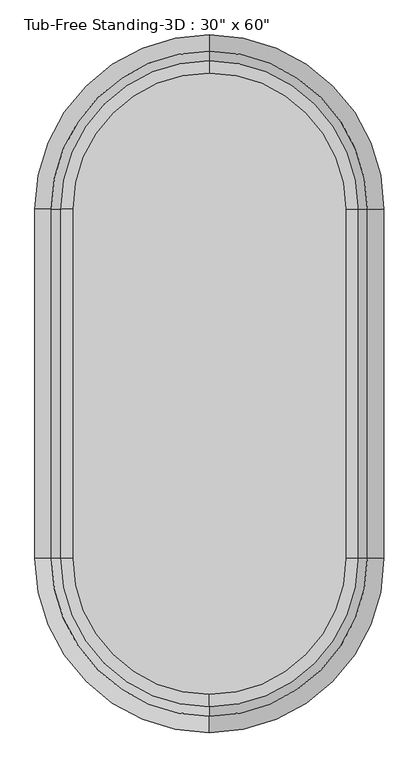
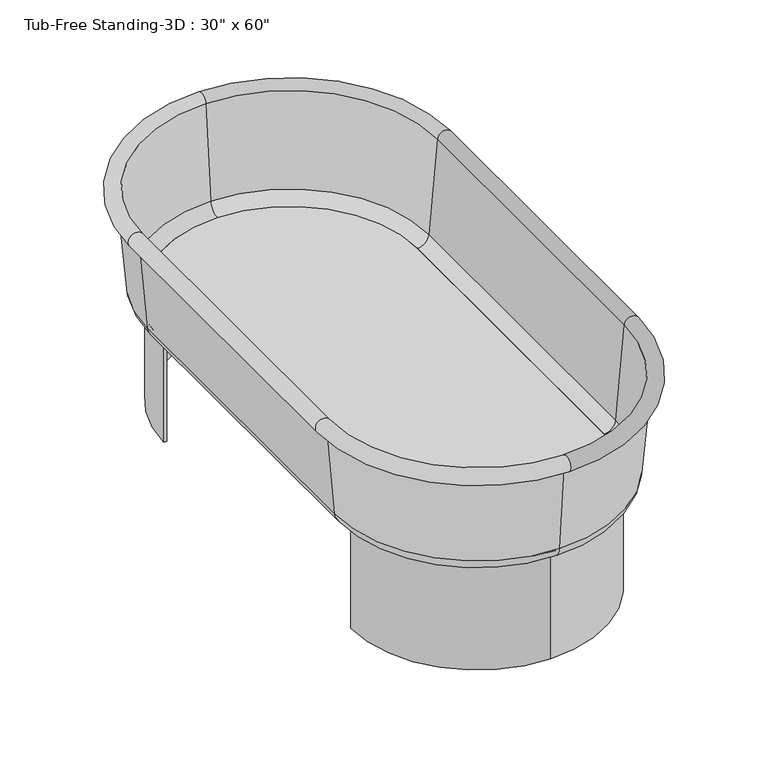
"""IFC4 building model written with IfcOpenShell, lengths in millimetres: flow terminal geometry."""

from ifc_helpers import new_model, si_unit, point, frame, frame_2d, origin, origin_with_axes, place, context, project, spatial, polyline, circle_curve, ellipse_curve, trimmed, segment, composite_curve, outline, extrude, source, transform, mapped, element, save
from ifc_brep_helpers import plane_surface, cylinder_surface, revolved_surface, advanced_brep


def flow_terminal_b46ab875(model_context):
    return source(origin(), model_context, "Body", "SolidModel", [
        extrude(outline(composite_curve([segment(trimmed(circle_curve(frame_2d((0.0, 533.4)), 406.4), [point((0.0, 939.8))], [point((-406.4, 533.4))], True, "CARTESIAN"), True, "CONTINUOUS"), segment(polyline([(-406.4, 533.4), (-416.6824236, 533.4)]), True, "CONTINUOUS"), segment(trimmed(circle_curve(frame_2d((0.0, 533.4)), 416.6824236), [point((-416.6824236, 533.4))], [point((0.0, 950.0824236))], False, "CARTESIAN"), True, "CONTINUOUS"), segment(trimmed(circle_curve(frame_2d((0.0, 533.4)), 416.6824236), [point((0.0, 950.0824236))], [point((416.6824236, 533.4))], False, "CARTESIAN"), True, "CONTINUOUS"), segment(polyline([(416.6824236, 533.4), (406.4, 533.4)]), True, "CONTINUOUS"), segment(trimmed(circle_curve(frame_2d((0.0, 533.4)), 406.4), [point((406.4, 533.4))], [point((0.0, 939.8))], True, "CARTESIAN"), True, "CONTINUOUS")], self_intersect=False)), origin_with_axes(), (0.0, 0.0, 1.0), 368.3),
        extrude(outline(composite_curve([segment(trimmed(circle_curve(frame_2d((0.0, -533.4)), 416.6824236), [point((0.0, -950.0824236))], [point((-416.6824236, -533.4))], False, "CARTESIAN"), True, "CONTINUOUS"), segment(polyline([(-416.6824236, -533.4), (-406.4, -533.4)]), True, "CONTINUOUS"), segment(trimmed(circle_curve(frame_2d((0.0, -533.4)), 406.4), [point((-406.4, -533.4))], [point((0.0, -939.8))], True, "CARTESIAN"), True, "CONTINUOUS"), segment(trimmed(circle_curve(frame_2d((0.0, -533.4)), 406.4), [point((0.0, -939.8))], [point((406.4, -533.4))], True, "CARTESIAN"), True, "CONTINUOUS"), segment(polyline([(406.4, -533.4), (416.6824236, -533.4)]), True, "CONTINUOUS"), segment(trimmed(circle_curve(frame_2d((0.0, -533.4)), 416.6824236), [point((416.6824236, -533.4))], [point((0.0, -950.0824236))], False, "CARTESIAN"), True, "CONTINUOUS")], self_intersect=False)), origin_with_axes(), (0.0, 0.0, 1.0), 368.3),
        extrude(outline(composite_curve([segment(polyline([(-416.6824236, -533.4), (-416.6824236, 533.4)]), True, "CONTINUOUS"), segment(trimmed(circle_curve(frame_2d((0.0, 533.4)), 416.6824236), [point((-416.6824236, 533.4))], [point((0.0, 950.0824236))], False, "CARTESIAN"), True, "CONTINUOUS"), segment(trimmed(circle_curve(frame_2d((0.0, 533.4)), 416.6824236), [point((0.0, 950.0824236))], [point((416.6824236, 533.4))], False, "CARTESIAN"), True, "CONTINUOUS"), segment(polyline([(416.6824236, 533.4), (416.6824236, -533.4)]), True, "CONTINUOUS"), segment(trimmed(circle_curve(frame_2d((0.0, -533.4)), 416.6824236), [point((416.6824236, -533.4))], [point((0.0, -950.0824236))], False, "CARTESIAN"), True, "CONTINUOUS"), segment(trimmed(circle_curve(frame_2d((0.0, -533.4)), 416.6824236), [point((0.0, -950.0824236))], [point((-416.6824236, -533.4))], False, "CARTESIAN"), True, "CONTINUOUS")], self_intersect=False)), frame((0.0, 0.0, 368.3), z_axis=(0.0, 0.0, 1.0), x_axis=(1.0, 0.0, 0.0)), (0.0, 0.0, 1.0), 15.08125),
        advanced_brep(
        [(0.0, -1028.7, 711.2), (495.3, -533.4, 711.2), (508.0, -533.4, 711.2), (0.0, -1041.4, 711.2), (0.0, -1002.9045038, 416.3561295), (469.5045038, -533.4, 416.3561295), (0.0, -950.0824236, 367.9536107), (416.6824236, -533.4, 367.9536107), (0.0, -950.0824236, 382.8774627), (416.6824236, -533.4, 382.8774627), (0.0, -988.0374416, 417.6568289), (454.6374416, -533.4, 417.6568289), (0.0, -1016.2561556, 740.1982063), (482.8561556, -533.4, 740.1982063), (-495.3, -533.4, 711.2), (-508.0, -533.4, 711.2), (-469.5045038, -533.4, 416.3561295), (-416.6824236, -533.4, 367.9536107), (-416.6824236, -533.4, 382.8774627), (-454.6374416, -533.4, 417.6568289), (-482.8561556, -533.4, 740.1982063), (-508.0, 533.4, 711.2), (-495.3, 533.4, 711.2), (-469.5045038, 533.4, 416.3561295), (-416.6824236, 533.4, 367.9536107), (-416.6824236, 533.4, 382.8774627), (-454.6374416, 533.4, 417.6568289), (-482.8561556, 533.4, 740.1982063), (0.0, 1028.7, 711.2), (0.0, 1041.4, 711.2), (0.0, 1002.9045038, 416.3561295), (0.0, 950.0824236, 367.9536107), (0.0, 950.0824236, 382.8774627), (0.0, 988.0374416, 417.6568289), (0.0, 1016.2561556, 740.1982063), (495.3, 533.4, 711.2), (508.0, 533.4, 711.2), (469.5045038, 533.4, 416.3561295), (416.6824236, 533.4, 367.9536107), (416.6824236, 533.4, 382.8774627), (454.6374416, 533.4, 417.6568289), (482.8561556, 533.4, 740.1982063)],
        [
            (0, 1, circle_curve(frame((0.0, -533.4, 711.2), z_axis=(0.0, 0.0, 1.0), x_axis=(1.0, 0.0, 0.0)), 495.3)),
            (1, 2),
            (2, 3, circle_curve(frame((0.0, -533.4, 711.2), z_axis=(0.0, 0.0, -1.0), x_axis=(1.0, 0.0, 0.0)), 508.0)),
            (3, 0),
            (4, 5, circle_curve(frame((0.0, -533.4, 416.3561295), z_axis=(0.0, 0.0, 1.0), x_axis=(1.0, 0.0, 0.0)), 469.5045038)),
            (5, 1),
            (0, 4),
            (6, 7, circle_curve(frame((0.0, -533.4, 367.9536107), z_axis=(0.0, 0.0, 1.0), x_axis=(1.0, 0.0, 0.0)), 416.6824236)),
            (7, 5, circle_curve(frame((416.6824236, -533.4, 420.9774627), z_axis=(0.0, -1.0, 0.0), x_axis=(1.0, 0.0, 0.0)), 53.023852)),
            (4, 6, circle_curve(frame((0.0, -950.0824236, 420.9774627), z_axis=(1.0, 0.0, 0.0), x_axis=(0.0, -1.0, 0.0)), 53.023852)),
            (8, 9, circle_curve(frame((0.0, -533.4, 382.8774627), z_axis=(0.0, 0.0, 1.0), x_axis=(1.0, 0.0, 0.0)), 416.6824236)),
            (9, 7),
            (6, 8),
            (10, 11, circle_curve(frame((0.0, -533.4, 417.6568289), z_axis=(0.0, 0.0, 1.0), x_axis=(1.0, 0.0, 0.0)), 454.6374416)),
            (11, 9, circle_curve(frame((416.6824236, -533.4, 420.9774627), z_axis=(0.0, 1.0, 0.0), x_axis=(1.0, 0.0, 0.0)), 38.1)),
            (8, 10, circle_curve(frame((0.0, -950.0824236, 420.9774627), z_axis=(-1.0, 0.0, 0.0), x_axis=(0.0, -1.0, 0.0)), 38.1)),
            (12, 13, circle_curve(frame((0.0, -533.4, 740.1982063), z_axis=(0.0, 0.0, 1.0), x_axis=(1.0, 0.0, 0.0)), 482.8561556)),
            (13, 11),
            (10, 12),
            (2, 13, circle_curve(frame((508.0, -533.4, 736.6), z_axis=(0.0, -1.0, 0.0), x_axis=(1.0, 0.0, 0.0)), 25.4)),
            (12, 3, circle_curve(frame((0.0, -1041.4, 736.6), z_axis=(1.0, 0.0, 0.0), x_axis=(0.0, -1.0, 0.0)), 25.4)),
            (14, 0, circle_curve(frame((0.0, -533.4, 711.2), z_axis=(0.0, 0.0, 1.0), x_axis=(0.0, -1.0, 0.0)), 495.3)),
            (3, 15, circle_curve(frame((0.0, -533.4, 711.2), z_axis=(0.0, 0.0, -1.0), x_axis=(0.0, -1.0, 0.0)), 508.0)),
            (15, 14),
            (16, 4, circle_curve(frame((0.0, -533.4, 416.3561295), z_axis=(0.0, 0.0, 1.0), x_axis=(0.0, -1.0, 0.0)), 469.5045038)),
            (14, 16),
            (17, 6, circle_curve(frame((0.0, -533.4, 367.9536107), z_axis=(0.0, 0.0, 1.0), x_axis=(0.0, -1.0, 0.0)), 416.6824236)),
            (16, 17, circle_curve(frame((-416.6824236, -533.4, 420.9774627), z_axis=(0.0, -1.0, 0.0), x_axis=(-1.0, 0.0, 0.0)), 53.023852)),
            (18, 8, circle_curve(frame((0.0, -533.4, 382.8774627), z_axis=(0.0, 0.0, 1.0), x_axis=(0.0, -1.0, 0.0)), 416.6824236)),
            (17, 18),
            (19, 10, circle_curve(frame((0.0, -533.4, 417.6568289), z_axis=(0.0, 0.0, 1.0), x_axis=(0.0, -1.0, 0.0)), 454.6374416)),
            (18, 19, circle_curve(frame((-416.6824236, -533.4, 420.9774627), z_axis=(0.0, 1.0, 0.0), x_axis=(-1.0, 0.0, 0.0)), 38.1)),
            (20, 12, circle_curve(frame((0.0, -533.4, 740.1982063), z_axis=(0.0, 0.0, 1.0), x_axis=(0.0, -1.0, 0.0)), 482.8561556)),
            (19, 20),
            (20, 15, circle_curve(frame((-508.0, -533.4, 736.6), z_axis=(0.0, -1.0, 0.0), x_axis=(-1.0, 0.0, 0.0)), 25.4)),
            (15, 21),
            (21, 22),
            (22, 14),
            (22, 23),
            (23, 16),
            (23, 24, circle_curve(frame((-416.6824236, 533.4, 420.9774627), z_axis=(0.0, -1.0, 0.0), x_axis=(-1.0, 0.0, 0.0)), 53.023852)),
            (24, 17),
            (24, 25),
            (25, 18),
            (25, 26, circle_curve(frame((-416.6824236, 533.4, 420.9774627), z_axis=(0.0, 1.0, 0.0), x_axis=(-1.0, 0.0, 0.0)), 38.1)),
            (26, 19),
            (26, 27),
            (27, 20),
            (27, 21, circle_curve(frame((-508.0, 533.4, 736.6), z_axis=(0.0, -1.0, 0.0), x_axis=(-1.0, 0.0, 0.0)), 25.4)),
            (28, 22, circle_curve(frame((0.0, 533.4, 711.2), z_axis=(0.0, 0.0, 1.0), x_axis=(-1.0, 0.0, 0.0)), 495.3)),
            (21, 29, circle_curve(frame((0.0, 533.4, 711.2), z_axis=(0.0, 0.0, -1.0), x_axis=(-1.0, 0.0, 0.0)), 508.0)),
            (29, 28),
            (30, 23, circle_curve(frame((0.0, 533.4, 416.3561295), z_axis=(0.0, 0.0, 1.0), x_axis=(-1.0, 0.0, 0.0)), 469.5045038)),
            (28, 30),
            (31, 24, circle_curve(frame((0.0, 533.4, 367.9536107), z_axis=(0.0, 0.0, 1.0), x_axis=(-1.0, 0.0, 0.0)), 416.6824236)),
            (30, 31, circle_curve(frame((0.0, 950.0824236, 420.9774627), z_axis=(-1.0, 0.0, 0.0), x_axis=(0.0, 1.0, 0.0)), 53.023852)),
            (32, 25, circle_curve(frame((0.0, 533.4, 382.8774627), z_axis=(0.0, 0.0, 1.0), x_axis=(-1.0, 0.0, 0.0)), 416.6824236)),
            (31, 32),
            (33, 26, circle_curve(frame((0.0, 533.4, 417.6568289), z_axis=(0.0, 0.0, 1.0), x_axis=(-1.0, 0.0, 0.0)), 454.6374416)),
            (32, 33, circle_curve(frame((0.0, 950.0824236, 420.9774627), z_axis=(1.0, 0.0, 0.0), x_axis=(0.0, 1.0, 0.0)), 38.1)),
            (34, 27, circle_curve(frame((0.0, 533.4, 740.1982063), z_axis=(0.0, 0.0, 1.0), x_axis=(-1.0, 0.0, 0.0)), 482.8561556)),
            (33, 34),
            (34, 29, circle_curve(frame((0.0, 1041.4, 736.6), z_axis=(-1.0, 0.0, 0.0), x_axis=(0.0, 1.0, 0.0)), 25.4)),
            (35, 28, circle_curve(frame((0.0, 533.4, 711.2), z_axis=(0.0, 0.0, 1.0), x_axis=(0.0, 1.0, 0.0)), 495.3)),
            (29, 36, circle_curve(frame((0.0, 533.4, 711.2), z_axis=(0.0, 0.0, -1.0), x_axis=(0.0, 1.0, 0.0)), 508.0)),
            (36, 35),
            (37, 30, circle_curve(frame((0.0, 533.4, 416.3561295), z_axis=(0.0, 0.0, 1.0), x_axis=(0.0, 1.0, 0.0)), 469.5045038)),
            (35, 37),
            (38, 31, circle_curve(frame((0.0, 533.4, 367.9536107), z_axis=(0.0, 0.0, 1.0), x_axis=(0.0, 1.0, 0.0)), 416.6824236)),
            (37, 38, circle_curve(frame((416.6824236, 533.4, 420.9774627), z_axis=(0.0, 1.0, 0.0), x_axis=(1.0, 0.0, 0.0)), 53.023852)),
            (39, 32, circle_curve(frame((0.0, 533.4, 382.8774627), z_axis=(0.0, 0.0, 1.0), x_axis=(0.0, 1.0, 0.0)), 416.6824236)),
            (38, 39),
            (40, 33, circle_curve(frame((0.0, 533.4, 417.6568289), z_axis=(0.0, 0.0, 1.0), x_axis=(0.0, 1.0, 0.0)), 454.6374416)),
            (39, 40, circle_curve(frame((416.6824236, 533.4, 420.9774627), z_axis=(0.0, -1.0, 0.0), x_axis=(1.0, 0.0, 0.0)), 38.1)),
            (41, 34, circle_curve(frame((0.0, 533.4, 740.1982063), z_axis=(0.0, 0.0, 1.0), x_axis=(0.0, 1.0, 0.0)), 482.8561556)),
            (40, 41),
            (41, 36, circle_curve(frame((508.0, 533.4, 736.6), z_axis=(0.0, 1.0, 0.0), x_axis=(1.0, 0.0, 0.0)), 25.4)),
            (36, 2),
            (1, 35),
            (5, 37),
            (7, 38),
            (9, 39),
            (11, 40),
            (13, 41),
        ],
        [
            plane_surface(frame((0.0, -533.4, 711.2), z_axis=(0.0, 0.0, -1.0), x_axis=(1.0, 0.0, 0.0))),
            revolved_surface(polyline([(495.3, -533.4, 711.2), (469.5045038, -533.4, 416.3561295)]), (0.0, -533.4, 736.6), (0.0, 0.0, -1.0)),
            revolved_surface(trimmed(ellipse_curve(frame((416.6824236, -533.4, 420.9774627), z_axis=(0.0, 1.0, 0.0), x_axis=(1.0, 0.0, 0.0)), 53.023852, 53.023852), [point((469.5045038, -533.4, 416.3561295))], [point((416.6824236, -533.4, 367.9536107))], True, "CARTESIAN"), (0.0, -533.4, 736.6), (0.0, 0.0, -1.0)),
            revolved_surface(polyline([(416.6824236, -533.4, 367.9536107), (416.6824236, -533.4, 382.8774627)]), (0.0, -533.4, 736.6), (0.0, 0.0, -1.0)),
            revolved_surface(trimmed(ellipse_curve(frame((416.6824236, -533.4, 420.9774627), z_axis=(0.0, -1.0, 0.0), x_axis=(1.0, 0.0, 0.0)), 38.1, 38.1), [point((416.6824236, -533.4, 382.8774627))], [point((454.6374416, -533.4, 417.6568289))], True, "CARTESIAN"), (0.0, -533.4, 736.6), (0.0, 0.0, -1.0)),
            revolved_surface(polyline([(454.6374416, -533.4, 417.6568289), (482.8561556, -533.4, 740.1982063)]), (0.0, -533.4, 736.6), (0.0, 0.0, -1.0)),
            revolved_surface(trimmed(ellipse_curve(frame((508.0, -533.4, 736.6), z_axis=(0.0, 1.0, 0.0), x_axis=(1.0, 0.0, 0.0)), 25.4, 25.4), [point((482.8561556, -533.4, 740.1982063))], [point((508.0, -533.4, 711.2))], True, "CARTESIAN"), (0.0, -533.4, 736.6), (0.0, 0.0, -1.0)),
            plane_surface(frame((0.0, -533.4, 711.2), z_axis=(0.0, 0.0, -1.0), x_axis=(0.0, -1.0, 0.0))),
            revolved_surface(polyline([(0.0, -1028.7, 711.2), (0.0, -1002.9045038, 416.3561295)]), (0.0, -533.4, 736.6), (0.0, 0.0, -1.0)),
            revolved_surface(trimmed(ellipse_curve(frame((0.0, -950.0824236, 420.9774627), z_axis=(1.0, 0.0, 0.0), x_axis=(0.0, -1.0, 0.0)), 53.023852, 53.023852), [point((0.0, -1002.9045038, 416.3561295))], [point((0.0, -950.0824236, 367.9536107))], True, "CARTESIAN"), (0.0, -533.4, 736.6), (0.0, 0.0, -1.0)),
            revolved_surface(polyline([(0.0, -950.0824236, 367.9536107), (0.0, -950.0824236, 382.8774627)]), (0.0, -533.4, 736.6), (0.0, 0.0, -1.0)),
            revolved_surface(trimmed(ellipse_curve(frame((0.0, -950.0824236, 420.9774627), z_axis=(-1.0, 0.0, 0.0), x_axis=(0.0, -1.0, 0.0)), 38.1, 38.1), [point((0.0, -950.0824236, 382.8774627))], [point((0.0, -988.0374416, 417.6568289))], True, "CARTESIAN"), (0.0, -533.4, 736.6), (0.0, 0.0, -1.0)),
            revolved_surface(polyline([(0.0, -988.0374416, 417.6568289), (0.0, -1016.2561556, 740.1982063)]), (0.0, -533.4, 736.6), (0.0, 0.0, -1.0)),
            revolved_surface(trimmed(ellipse_curve(frame((0.0, -1041.4, 736.6), z_axis=(1.0, 0.0, 0.0), x_axis=(0.0, -1.0, 0.0)), 25.4, 25.4), [point((0.0, -1016.2561556, 740.1982063))], [point((0.0, -1041.4, 711.2))], True, "CARTESIAN"), (0.0, -533.4, 736.6), (0.0, 0.0, -1.0)),
            plane_surface(frame((-508.0, -533.4, 711.2), z_axis=(0.0, 0.0, -1.0), x_axis=(0.0, 1.0, 0.0))),
            plane_surface(frame((-495.3, -533.4, 711.2), z_axis=(-0.9961946980917455, 0.0, -0.0871557427476588), x_axis=(0.0, 1.0, 0.0))),
            cylinder_surface(frame((-416.6824236, -533.4, 420.9774627), z_axis=(0.0, -1.0, 0.0), x_axis=(-1.0, 0.0, 0.0)), 53.023852),
            plane_surface(frame((-416.6824236, -533.4, 367.9536107), z_axis=(1.0, 0.0, 0.0), x_axis=(0.0, 1.0, 0.0))),
            revolved_surface(polyline([(-454.7824236, 533.4, 420.9774627), (-454.7824236, -533.4, 420.9774627)]), (-416.6824236, -533.4, 420.9774627), (0.0, 1.0, 0.0)),
            plane_surface(frame((-454.6374416, -533.4, 417.6568289), z_axis=(0.9961946980917457, 0.0, 0.08715574274765674), x_axis=(0.0, 1.0, 0.0))),
            cylinder_surface(frame((-508.0, -533.4, 736.6), z_axis=(0.0, -1.0, 0.0), x_axis=(-1.0, 0.0, 0.0)), 25.4),
            plane_surface(frame((0.0, 533.4, 711.2), z_axis=(0.0, 0.0, -1.0), x_axis=(-1.0, 0.0, 0.0))),
            revolved_surface(polyline([(-495.3, 533.4, 711.2), (-469.5045038, 533.4, 416.3561295)]), (0.0, 533.4, 736.6), (0.0, 0.0, -1.0)),
            revolved_surface(trimmed(ellipse_curve(frame((-416.6824236, 533.4, 420.9774627), z_axis=(0.0, -1.0, 0.0), x_axis=(-1.0, 0.0, 0.0)), 53.023852, 53.023852), [point((-469.5045038, 533.4, 416.3561295))], [point((-416.6824236, 533.4, 367.9536107))], True, "CARTESIAN"), (0.0, 533.4, 736.6), (0.0, 0.0, -1.0)),
            revolved_surface(polyline([(-416.6824236, 533.4, 367.9536107), (-416.6824236, 533.4, 382.8774627)]), (0.0, 533.4, 736.6), (0.0, 0.0, -1.0)),
            revolved_surface(trimmed(ellipse_curve(frame((-416.6824236, 533.4, 420.9774627), z_axis=(0.0, 1.0, 0.0), x_axis=(-1.0, 0.0, 0.0)), 38.1, 38.1), [point((-416.6824236, 533.4, 382.8774627))], [point((-454.6374416, 533.4, 417.6568289))], True, "CARTESIAN"), (0.0, 533.4, 736.6), (0.0, 0.0, -1.0)),
            revolved_surface(polyline([(-454.6374416, 533.4, 417.6568289), (-482.8561556, 533.4, 740.1982063)]), (0.0, 533.4, 736.6), (0.0, 0.0, -1.0)),
            revolved_surface(trimmed(ellipse_curve(frame((-508.0, 533.4, 736.6), z_axis=(0.0, -1.0, 0.0), x_axis=(-1.0, 0.0, 0.0)), 25.4, 25.4), [point((-482.8561556, 533.4, 740.1982063))], [point((-508.0, 533.4, 711.2))], True, "CARTESIAN"), (0.0, 533.4, 736.6), (0.0, 0.0, -1.0)),
            plane_surface(frame((0.0, 533.4, 711.2), z_axis=(0.0, 0.0, -1.0), x_axis=(0.0, 1.0, 0.0))),
            revolved_surface(polyline([(0.0, 1028.7, 711.2), (0.0, 1002.9045038, 416.3561295)]), (0.0, 533.4, 736.6), (0.0, 0.0, -1.0)),
            revolved_surface(trimmed(ellipse_curve(frame((0.0, 950.0824236, 420.9774627), z_axis=(-1.0, 0.0, 0.0), x_axis=(0.0, 1.0, 0.0)), 53.023852, 53.023852), [point((0.0, 1002.9045038, 416.3561295))], [point((0.0, 950.0824236, 367.9536107))], True, "CARTESIAN"), (0.0, 533.4, 736.6), (0.0, 0.0, -1.0)),
            revolved_surface(polyline([(0.0, 950.0824236, 367.9536107), (0.0, 950.0824236, 382.8774627)]), (0.0, 533.4, 736.6), (0.0, 0.0, -1.0)),
            revolved_surface(trimmed(ellipse_curve(frame((0.0, 950.0824236, 420.9774627), z_axis=(1.0, 0.0, 0.0), x_axis=(0.0, 1.0, 0.0)), 38.1, 38.1), [point((0.0, 950.0824236, 382.8774627))], [point((0.0, 988.0374416, 417.6568289))], True, "CARTESIAN"), (0.0, 533.4, 736.6), (0.0, 0.0, -1.0)),
            revolved_surface(polyline([(0.0, 988.0374416, 417.6568289), (0.0, 1016.2561556, 740.1982063)]), (0.0, 533.4, 736.6), (0.0, 0.0, -1.0)),
            revolved_surface(trimmed(ellipse_curve(frame((0.0, 1041.4, 736.6), z_axis=(-1.0, 0.0, 0.0), x_axis=(0.0, 1.0, 0.0)), 25.4, 25.4), [point((0.0, 1016.2561556, 740.1982063))], [point((0.0, 1041.4, 711.2))], True, "CARTESIAN"), (0.0, 533.4, 736.6), (0.0, 0.0, -1.0)),
            plane_surface(frame((508.0, 533.4, 711.2), z_axis=(0.0, 0.0, -1.0), x_axis=(0.0, -1.0, 0.0))),
            plane_surface(frame((495.3, 533.4, 711.2), z_axis=(0.9961946980917455, 0.0, -0.0871557427476588), x_axis=(0.0, -1.0, 0.0))),
            cylinder_surface(frame((416.6824236, 533.4, 420.9774627), z_axis=(0.0, 1.0, 0.0), x_axis=(1.0, 0.0, 0.0)), 53.023852),
            plane_surface(frame((416.6824236, 533.4, 367.9536107), z_axis=(-1.0, 0.0, 0.0), x_axis=(0.0, -1.0, 0.0))),
            revolved_surface(polyline([(454.7824236, -533.4, 420.9774627), (454.7824236, 533.4, 420.9774627)]), (416.6824236, 533.4, 420.9774627), (0.0, -1.0, 0.0)),
            plane_surface(frame((454.6374416, 533.4, 417.6568289), z_axis=(-0.9961946980917458, 0.0, 0.08715574274765675), x_axis=(0.0, -1.0, 0.0))),
            cylinder_surface(frame((508.0, 533.4, 736.6), z_axis=(0.0, 1.0, 0.0), x_axis=(1.0, 0.0, 0.0)), 25.4),
        ],
        [
            (0, [[1, 2, 3, 4]]),
            (1, [[5, 6, -1, 7]]),
            (2, [[8, 9, -5, 10]]),
            (3, [[11, 12, -8, 13]]),
            (4, [[14, 15, -11, 16]]),
            (5, [[17, 18, -14, 19]]),
            (6, [[-3, 20, -17, 21]]),
            (7, [[22, -4, 23, 24]]),
            (8, [[25, -7, -22, 26]]),
            (9, [[27, -10, -25, 28]]),
            (10, [[29, -13, -27, 30]]),
            (11, [[31, -16, -29, 32]]),
            (12, [[33, -19, -31, 34]]),
            (13, [[-23, -21, -33, 35]]),
            (14, [[-24, 36, 37, 38]]),
            (15, [[-26, -38, 39, 40]]),
            (16, [[-28, -40, 41, 42]]),
            (17, [[-30, -42, 43, 44]]),
            (18, [[-32, -44, 45, 46]]),
            (19, [[-34, -46, 47, 48]]),
            (20, [[-35, -48, 49, -36]]),
            (21, [[50, -37, 51, 52]]),
            (22, [[53, -39, -50, 54]]),
            (23, [[55, -41, -53, 56]]),
            (24, [[57, -43, -55, 58]]),
            (25, [[59, -45, -57, 60]]),
            (26, [[61, -47, -59, 62]]),
            (27, [[-51, -49, -61, 63]]),
            (28, [[64, -52, 65, 66]]),
            (29, [[67, -54, -64, 68]]),
            (30, [[69, -56, -67, 70]]),
            (31, [[71, -58, -69, 72]]),
            (32, [[73, -60, -71, 74]]),
            (33, [[75, -62, -73, 76]]),
            (34, [[-65, -63, -75, 77]]),
            (35, [[-66, 78, -2, 79]]),
            (36, [[-68, -79, -6, 80]]),
            (37, [[-70, -80, -9, 81]]),
            (38, [[-72, -81, -12, 82]]),
            (39, [[-74, -82, -15, 83]]),
            (40, [[-76, -83, -18, 84]]),
            (41, [[-77, -84, -20, -78]]),
        ],
    ),
    ])


if __name__ == "__main__":
    model = new_model("IFC4")
    model_context = context("Model", 3, world=origin())
    ifc_project = project(units=[si_unit("LENGTHUNIT", "METRE", prefix="MILLI")], contexts=[model_context])
    site = spatial("IfcSite", under=ifc_project)
    building = spatial("IfcBuilding", under=site)
    placement = place(None, origin())
    flow_terminal_shape = flow_terminal_b46ab875(model_context)
    element("IfcFlowTerminal", 1, ObjectType="Tub-Free Standing-3D : 30\" x 60\"", at=placement, inside=building, context=model_context, shape_type="MappedRepresentation", body=[
        mapped(flow_terminal_shape, transform((0.0, 0.0, 0.0), x_axis=(1.0, 0.0, 0.0), y_axis=(0.0, 1.0, 0.0), z_axis=(0.0, 0.0, 1.0))),
    ])
    save(model, "model.ifc")

# Revit data of these elements
# Type "Tub-Free Standing-3D : 30\" x 60\""
#   Assembly Code = "D2010110"
#   Height = 2' - 6"
#   Length = 7' - 0"
#   Width = 3' - 6"
#   Tub Material = Porcelain, Ivory
#   Default Elevation = 0
# Element 1 (IfcFlowTerminal, "Tub-Free Standing-3D : 30\" x 60\"")
#   Materials on its faces: "Porcelain, Ivory"
# Materials
#   "Porcelain, Ivory": class "Ceramic", colour RGB 247 247 239, transparency 0, Description = "Porcelain, ivory", Cost = 0
